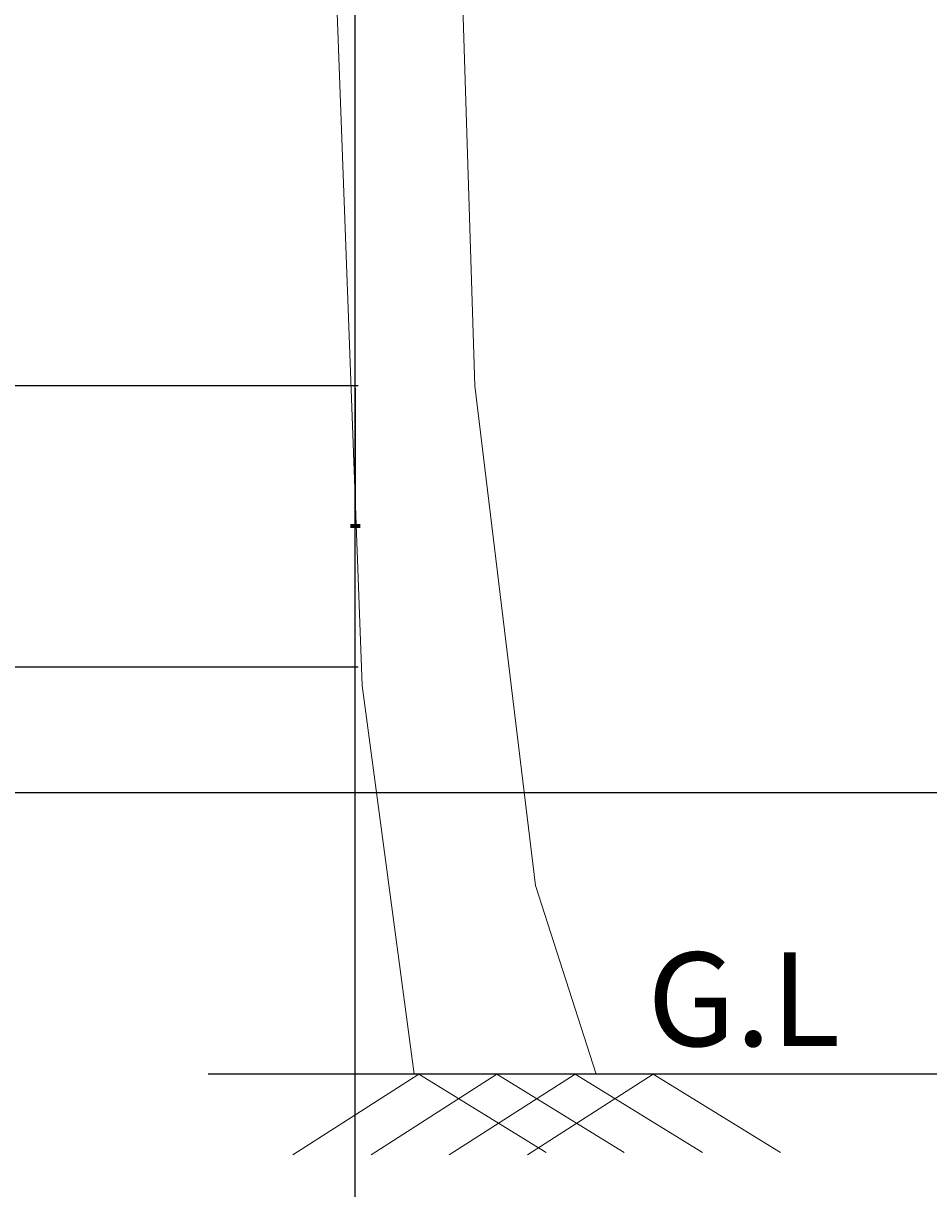
# Model space of a CAD drawing. Units: inches. Extents: x -301 to 715, y -607 to 364.
# Tile 127 of 141: x 194 to 252, y -515 to -440. Entities that reach past the tile are written whole.
import ezdxf

# ---------------------------------------------------------------- set-up
doc = ezdxf.new("R2010")
doc.units = ezdxf.units.IN
doc.header["$MEASUREMENT"] = 0
for name, color, linetype, lineweight in [('A-ANNO-DIMS', 2, 'Continuous', 18), ('A-ANNO-SYMB', 4, 'Continuous', 18), ('A-GRND', 7, 'Continuous', 25), ('L-PLNT', 94, 'Continuous', 13)]:
    doc.layers.add(name, color=color, linetype=linetype, lineweight=lineweight)
doc.styles.get("Standard").update_dxf_attribs({"font": 'arial.ttf'})
doc.dimstyles.get("Standard").update_dxf_attribs({"dimtxt": 0.18, "dimasz": 0.18, "dimexe": 0.18, "dimexo": 0.0625, "dimgap": 0.09, "dimtad": 0, "dimtih": 1, "dimtoh": 1, "dimdec": 1, "dimzin": 0, "dimdsep": 46, "dimlunit": 4, "dimtxsty": 'Standard', "dimcen": 0.09, "dimclrd": 3, "dimclre": 4, "dimclrt": 6, "dimadec": 0, "dimazin": 0, "dimtfac": 1, "dimtdec": 1, "dimtofl": 0, "dimtmove": 0, "dimatfit": 3, "dimfxl": 1, "dimtfill": 2, "dimtfillclr": 51, "dimtolj": 1, "dimtzin": 0, "dimarcsym": 0})

# ---------------------------------------------------------------- blocks, each defined once
blk = doc.blocks.new('*U34')
for points in [[(-2.363, 170.553), (-3.88, 148.505), (-4.988, 69.634), (-3.325, 24.869), (0, 0)], [(-0.116, 162.848), (0.554, 143.532), (2.217, 96.635), (3.88, 44.054), (7.76, 12.079), (11.64, 0)]]:
    blk.add_lwpolyline(points)
blk = doc.blocks.new('GRADE-MARK-4')
for p, q in [((8.05, 5.162), (0, 0)), ((13.05, 5.162), (5, 0)), ((8.05, 5.162), (16.196, 0.151)), ((18.05, 5.162), (10, 0)), ((13.05, 5.162), (21.196, 0.151)), ((23.05, 5.162), (15, 0)), ((18.05, 5.162), (26.196, 0.151)), ((23.05, 5.162), (31.196, 0.151))]:
    blk.add_line(p, q)
blk = doc.blocks.new('*D176')
at = {"layer": 'A-ANNO-DIMS', "color": 4, "lineweight": -2, "transparency": 16777216}
for p, q in [((148.28, -324.477), (215.605, -324.477)), ((-15.22, -540.477), (215.605, -540.477))]:
    blk.add_line(p, q, dxfattribs=at)
at = {"layer": 'A-ANNO-DIMS', "color": 3, "lineweight": -2, "transparency": 16777216}
for p, q in [((215.425, -324.657), (215.425, -432.296)), ((215.425, -540.297), (215.425, -432.659))]:
    blk.add_line(p, q, dxfattribs=at)
at = {"layer": 'A-ANNO-DIMS', "color": 3, "transparency": 16777216}
for points in [[(215.395, -324.657), (215.455, -324.657), (215.425, -324.477)], [(215.395, -540.297), (215.455, -540.297), (215.425, -540.477)]]:
    blk.add_solid(points, dxfattribs=at)
at = {"layer": 'Defpoints', "color": 0, "transparency": 16777216}
for p in [(148.218, -324.477), (-15.282, -540.477), (215.425, -540.477)]:
    blk.add_point(p, dxfattribs=at)
at = {"layer": 'A-ANNO-DIMS', "color": 6, "transparency": 16777216, "insert": (215.425, -432.477), "char_height": 0.18, "attachment_point": 5, "bg_fill": 1, "box_fill_scale": 1.25, "bg_fill_color": 51, "bg_fill_transparency": 0}
blk.add_mtext('\\A1;18\'-0"', dxfattribs=at)
blk = doc.blocks.new('*D188')
at = {"layer": 'A-ANNO-DIMS', "color": 4, "lineweight": -2, "transparency": 16777216}
for p, q in [((148.28, -463.477), (215.605, -463.477)), ((158.28, -481.477), (215.605, -481.477))]:
    blk.add_line(p, q, dxfattribs=at)
at = {"layer": 'A-ANNO-DIMS', "color": 3, "lineweight": -2, "transparency": 16777216}
for p, q in [((215.425, -463.657), (215.425, -472.296)), ((215.425, -481.297), (215.425, -472.659))]:
    blk.add_line(p, q, dxfattribs=at)
at = {"layer": 'A-ANNO-DIMS', "color": 3, "transparency": 16777216}
for points in [[(215.395, -463.657), (215.455, -463.657), (215.425, -463.477)], [(215.395, -481.297), (215.455, -481.297), (215.425, -481.477)]]:
    blk.add_solid(points, dxfattribs=at)
at = {"layer": 'Defpoints', "color": 0, "transparency": 16777216}
for p in [(148.218, -463.477), (215.425, -463.477), (158.218, -481.477)]:
    blk.add_point(p, dxfattribs=at)
at = {"layer": 'A-ANNO-DIMS', "color": 6, "transparency": 16777216, "insert": (215.425, -472.477), "char_height": 0.18, "attachment_point": 5, "bg_fill": 1, "box_fill_scale": 1.25, "bg_fill_color": 51, "bg_fill_transparency": 0}
blk.add_mtext('\\A1;1\'-6"', dxfattribs=at)
blk = doc.blocks.new('*D200')
at = {"layer": 'A-ANNO-DIMS', "color": 4, "lineweight": -2, "transparency": 16777216}
for p, q in [((412.955, -393.552), (121.926, -393.552)), ((412.955, -489.552), (121.926, -489.552))]:
    blk.add_line(p, q, dxfattribs=at)
at = {"layer": 'A-ANNO-DIMS', "color": 3, "lineweight": -2, "transparency": 16777216}
for p, q in [((122.106, -393.732), (122.106, -441.371)), ((122.106, -489.372), (122.106, -441.734))]:
    blk.add_line(p, q, dxfattribs=at)
at = {"layer": 'A-ANNO-DIMS', "color": 3, "transparency": 16777216}
for points in [[(122.076, -393.732), (122.136, -393.732), (122.106, -393.552)], [(122.076, -489.372), (122.136, -489.372), (122.106, -489.552)]]:
    blk.add_solid(points, dxfattribs=at)
at = {"layer": 'Defpoints', "color": 0, "transparency": 16777216}
for p in [(122.106, -393.552), (413.018, -393.552), (413.018, -489.552)]:
    blk.add_point(p, dxfattribs=at)
at = {"layer": 'A-ANNO-DIMS', "color": 6, "transparency": 16777216, "insert": (122.106, -441.552), "char_height": 0.18, "attachment_point": 5, "bg_fill": 1, "box_fill_scale": 1.25, "bg_fill_color": 51, "bg_fill_transparency": 0}
blk.add_mtext('\\A1;8\'-0"', dxfattribs=at)

msp = doc.modelspace()

# ---------------------------------------------------------------- linework, layer by layer
at = {"layer": 'A-GRND'}
msp.add_line((254.018, -507.552), (206.018, -507.552), dxfattribs=at)

# ---------------------------------------------------------------- block references
at = {"layer": 'A-ANNO-SYMB'}
msp.add_blockref('GRADE-MARK-4', (211.435, -512.714), dxfattribs=at)
at = {"layer": 'L-PLNT'}
msp.add_blockref('*U34', (219.184, -507.552), dxfattribs=at)

# ---------------------------------------------------------------- texts
at = {"layer": 'A-ANNO-SYMB'}
msp.add_text('G.L', height=6, dxfattribs=at).set_placement((234.103, -505.753))

# ---------------------------------------------------------------- dimensions: what is measured, and where the dimension line sits
at = {"layer": 'A-ANNO-DIMS'}
for base, p1, p2, picture, middle in [((215.425, -540.477), (148.218, -324.477), (-15.282, -540.477), '*D176', (215.425, -432.477)), ((122.106, -393.552), (413.018, -489.552), (413.018, -393.552), '*D200', (122.106, -441.552)), ((215.425, -463.477), (158.218, -481.477), (148.218, -463.477), '*D188', (215.425, -472.477))]:
    dim = msp.add_linear_dim(base=base, p1=p1, p2=p2, angle=90, dimstyle='Standard', override={"dimdec": 1, "dimlfac": 1, "dimrnd": 0, "dimzin": 1, "dimdsep": 46, "dimlunit": 4, "dimfrac": 2}, dxfattribs=at)
    dim.commit()
    dim.dimension.update_dxf_attribs({"geometry": picture, "text_midpoint": middle})

doc.saveas('drawing.dxf')
